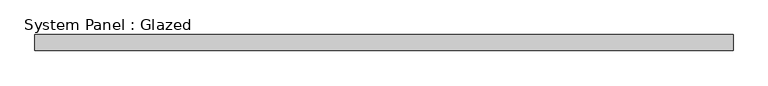
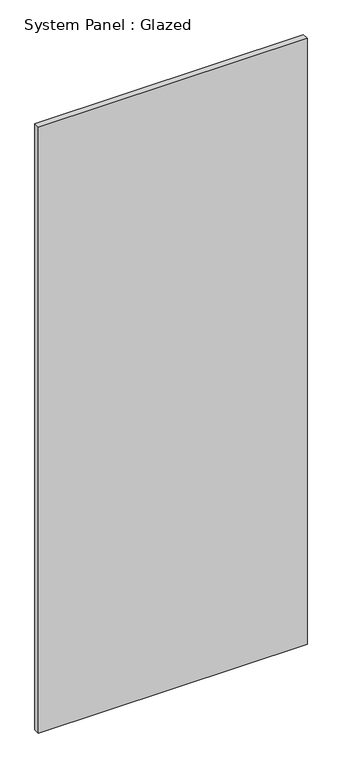
"""IFC4 building model written with IfcOpenShell, lengths in millimetres: plate geometry, System Panel : Glazed."""

from ifc_helpers import new_model, si_unit, origin, origin_with_axes, place, context, project, spatial, polyline, outline, extrude, source, transform, mapped, element, save


def system_panel_glazed_aebd10dd(model_context):
    return source(origin(), model_context, "Body", "SweptSolid", [
        extrude(outline(polyline([(555.3125873, 19.05), (-555.3125873, 19.05), (-555.3125873, 44.45), (555.3125873, 44.45), (555.3125873, 19.05)])), origin_with_axes(), (0.0, 0.0, 1.0), 2647.95),
    ])


if __name__ == "__main__":
    model = new_model("IFC4")
    model_context = context("Model", 3, world=origin())
    ifc_project = project(units=[si_unit("LENGTHUNIT", "METRE", prefix="MILLI")], contexts=[model_context])
    site = spatial("IfcSite", under=ifc_project)
    building = spatial("IfcBuilding", under=site)
    placement = place(None, origin())
    system_panel_glazed_shape = system_panel_glazed_aebd10dd(model_context)
    element("IfcPlate", 1, ObjectType="System Panel : Glazed", at=placement, inside=building, context=model_context, shape_type="MappedRepresentation", body=[
        mapped(system_panel_glazed_shape, transform((0.0, 0.0, 0.0), x_axis=(1.0, 0.0, 0.0), y_axis=(0.0, 1.0, 0.0), z_axis=(0.0, 0.0, 1.0))),
    ])
    save(model, "model.ifc")

# Revit data of these elements
# Type "System Panel : Glazed"
#   Construction Type Id = "GSP4R"
#   Analytic Construction = "1/8 in Pilkington single glazing"
#   Visual Light Transmittance = 0.9
#   Solar Heat Gain Coefficient = 0.86
#   Heat Transfer Coefficient (U) = 1.18115 BTU/(h·ft²·°F)
# Element 1 (IfcPlate, "System Panel : Glazed")
#   Materials on its faces: "Glass"
# Materials
#   "Glass": class "Glass", colour RGB 0 128 192, transparency 0.75, Description = "Soda Lime Glass", Cost = 0
